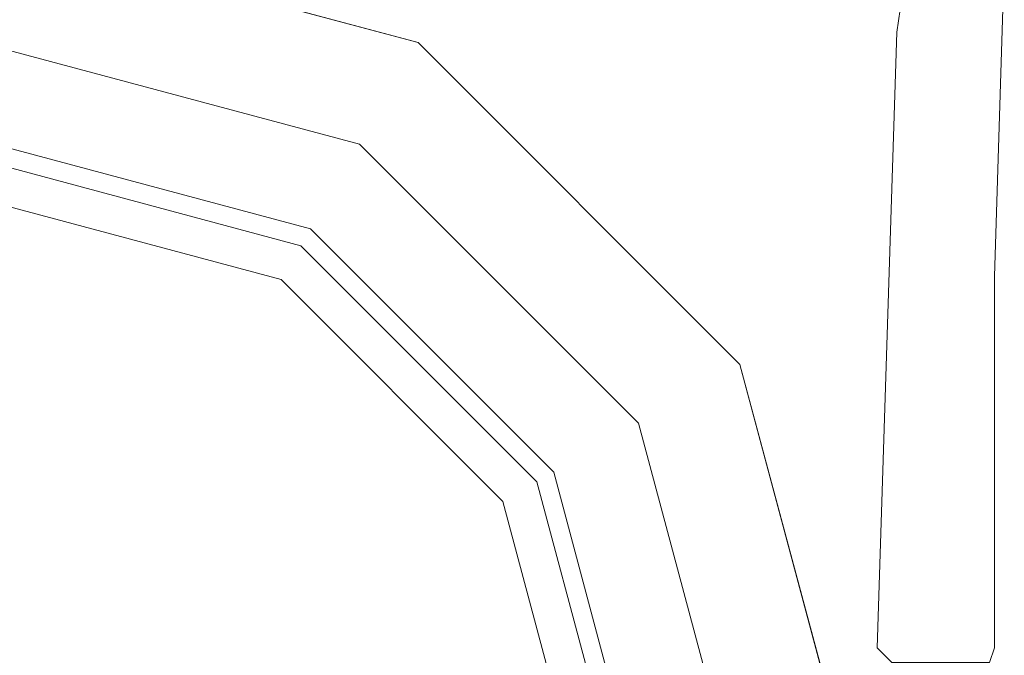
# Model space of a CAD drawing. Units: inches. Extents: x 375 to 1122, y 27 to 1069.
# Tile 12 of 155: x 725.941 to 732.144, y 262.679 to 266.682. Entities that reach past the tile are written whole.
import ezdxf

# ---------------------------------------------------------------- set-up
doc = ezdxf.new("R2010")
doc.units = ezdxf.units.IN
doc.layers.add('Furniture', color=30, linetype='Continuous', lineweight=18)

# ---------------------------------------------------------------- blocks, each defined once
blk = doc.blocks.new('A$C403C54AD')
for points, invisible_edges in [([(1.98174, 1.16457, -0.05399), (1.98174, 1.17996, -0.05399), (2.031, 1.17842, -0.05399), (1.99252, 1.16303, -0.05399)], 5), ([(1.98174, 1.16457, -0.05553), (1.98174, 1.17996, -0.05553), (2.031, 1.17842, -0.05553), (1.99252, 1.16303, -0.05553)], 5), ([(2.031, 1.17842, -0.05553), (2.031, 1.17842, -0.05399), (1.98174, 1.17996, -0.05399), (1.98174, 1.17996, -0.05553)], 5), ([(2.031, 1.17842, -0.05399), (1.99252, 1.16303, -0.05399), (2.08949, 1.15995, -0.05399), (2.08949, 1.17842, -0.05399)], 5), ([(2.031, 1.17842, -0.05553), (1.99252, 1.16303, -0.05553), (2.08949, 1.15995, -0.05553), (2.08949, 1.17842, -0.05553)], 5), ([(2.08949, 1.17842, -0.05399), (2.08949, 1.17842, -0.05553), (2.031, 1.17842, -0.05553), (2.031, 1.17842, -0.05399)], 5), ([(2.08949, 1.15995, -0.05399), (2.08949, 1.17842, -0.05399), (2.0918, 1.17765, -0.05322), (2.0918, 1.16226, -0.05322)], 1), ([(2.08949, 1.15995, -0.05553), (2.08949, 1.17842, -0.05553), (2.0918, 1.17765, -0.0563), (2.0918, 1.16226, -0.0563)], 1), ([(2.0918, 1.17765, -0.0563), (2.0918, 1.17765, -0.05322), (2.08949, 1.17842, -0.05399), (2.08949, 1.17842, -0.05553)], 5), ([(1.98174, 1.16457, -0.05399), (1.98174, 1.16457, -0.05553), (1.99252, 1.16303, -0.05553), (1.99252, 1.16303, -0.05399)], 5), ([(1.99252, 1.16303, -0.05553), (1.99252, 1.16303, -0.05399), (2.08949, 1.15995, -0.05399), (2.08949, 1.15995, -0.05553)], 5), ([(2.08949, 1.15995, -0.05553), (2.08949, 1.15995, -0.05399), (2.0918, 1.16226, -0.05322), (2.0918, 1.16226, -0.0563)], 5)]:
    blk.add_3dface(points, dxfattribs=dict(invisible_edges=invisible_edges))
at = {"linetype": 'ByBlock', "invisible_edges": 5}
for points in [[(2.11411, 1.15687, -0.03783), (2.11411, 1.1384, -0.03783), (2.05409, 1.12232, -0.03783), (2.04485, 1.13831, -0.03783)], [(2.11411, 1.12301, -0.05168), (2.11411, 1.15687, -0.04244), (2.04485, 1.13831, -0.04244), (2.06178, 1.10899, -0.05168)], [(2.11411, 1.1384, -0.03783), (2.11411, 1.11993, -0.04398), (2.06332, 1.10632, -0.04398), (2.05409, 1.12232, -0.03783)], [(2.04485, 1.13831, -0.03783), (2.05409, 1.12232, -0.03783), (2.01014, 1.07837, -0.03783), (1.99415, 1.08761, -0.03783)], [(2.06178, 1.10899, -0.05168), (2.04485, 1.13831, -0.04244), (1.99415, 1.08761, -0.04244), (2.02347, 1.07068, -0.05168)], [(2.11411, 1.11377, -0.06091), (2.11411, 1.12301, -0.05168), (2.06178, 1.10899, -0.05168), (2.0664, 1.10099, -0.06091)], [(2.05409, 1.12232, -0.03783), (2.06332, 1.10632, -0.04398), (2.02614, 1.06914, -0.04398), (2.01014, 1.07837, -0.03783)], [(2.11411, 1.11993, -0.04398), (2.11411, 1.01834, -0.04398), (2.11411, 1.01834, -0.04398), (2.06332, 1.10632, -0.04398)], [(2.0664, 1.10099, -0.06091), (2.06178, 1.10899, -0.05168), (2.02347, 1.07068, -0.05168), (2.03147, 1.06606, -0.06091)], [(2.06332, 1.10632, -0.04398), (2.11411, 1.01834, -0.04398), (2.11411, 1.01834, -0.04398), (2.02614, 1.06914, -0.04398)], [(1.99415, 1.08761, -0.03783), (2.01014, 1.07837, -0.03783), (1.99406, 1.01834, -0.03783), (1.97559, 1.01834, -0.03783)], [(2.02347, 1.07068, -0.05168), (1.99415, 1.08761, -0.04244), (1.97559, 1.01834, -0.04244), (2.00945, 1.01834, -0.05168)], [(2.01014, 1.07837, -0.03783), (2.02614, 1.06914, -0.04398), (2.01253, 1.01834, -0.04398), (1.99406, 1.01834, -0.03783)], [(2.03147, 1.06606, -0.06091), (2.02347, 1.07068, -0.05168), (2.00945, 1.01834, -0.05168), (2.01868, 1.01834, -0.06091)], [(2.02614, 1.06914, -0.04398), (2.11411, 1.01834, -0.04398), (2.11411, 1.01834, -0.04398), (2.01253, 1.01834, -0.04398)]]:
    blk.add_3dface(points, dxfattribs=at)
at = {"linetype": 'ByBlock'}
for points in [[(2.11411, 1.15687, -0.04244), (2.11411, 1.15687, -0.03783), (2.04485, 1.13831, -0.03783), (2.04485, 1.13831, -0.04244)], [(2.04485, 1.13831, -0.04244), (2.04485, 1.13831, -0.03783), (1.99415, 1.08761, -0.03783), (1.99415, 1.08761, -0.04244)], [(1.99415, 1.08761, -0.04244), (1.99415, 1.08761, -0.03783), (1.97559, 1.01834, -0.03783), (1.97559, 1.01834, -0.04244)]]:
    blk.add_3dface(points, dxfattribs=at)

msp = doc.modelspace()

# ---------------------------------------------------------------- block references
at = {"layer": 'Furniture', "xscale": 39.9918517141215, "yscale": 39.9918517141215, "zscale": 39.9918517141215, "rotation": 270}
msp.add_blockref('A$C403C54AD', (684.9549, 346.2875, 0.024), dxfattribs=at)

doc.saveas('drawing.dxf')
